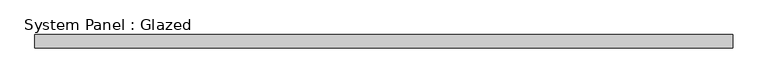
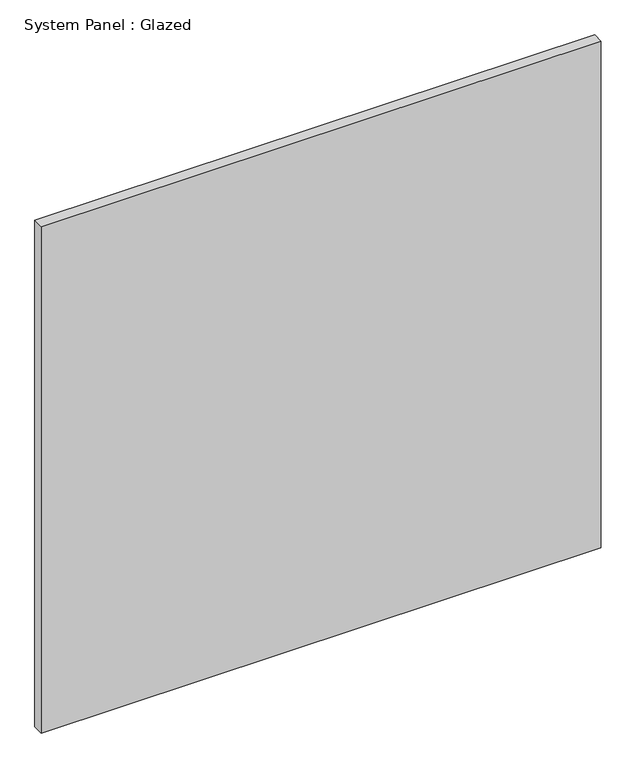
"""IFC4 building model written with IfcOpenShell, lengths in millimetres: plate geometry, System Panel : Glazed."""

from ifc_helpers import new_model, si_unit, origin, origin_with_axes, place, context, project, spatial, polyline, outline, extrude, source, transform, mapped, element, save


def system_panel_glazed_7e5d82eb(model_context):
    return source(origin(), model_context, "Body", "SweptSolid", [
        extrude(outline(polyline([(667.8083334, 19.05), (-667.8083334, 19.05), (-667.8083334, 44.45), (667.8083334, 44.45), (667.8083334, 19.05)])), origin_with_axes(), (0.0, 0.0, 1.0), 1276.35),
    ])


if __name__ == "__main__":
    model = new_model("IFC4")
    model_context = context("Model", 3, world=origin())
    ifc_project = project(units=[si_unit("LENGTHUNIT", "METRE", prefix="MILLI")], contexts=[model_context])
    site = spatial("IfcSite", under=ifc_project)
    building = spatial("IfcBuilding", under=site)
    placement = place(None, origin())
    system_panel_glazed_shape = system_panel_glazed_7e5d82eb(model_context)
    element("IfcPlate", 1, ObjectType="System Panel : Glazed", at=placement, inside=building, context=model_context, shape_type="MappedRepresentation", body=[
        mapped(system_panel_glazed_shape, transform((0.0, 0.0, 0.0), x_axis=(1.0, 0.0, 0.0), y_axis=(0.0, 1.0, 0.0), z_axis=(0.0, 0.0, 1.0))),
    ])
    save(model, "model.ifc")

# Revit data of these elements
# Type "System Panel : Glazed"
#   Construction Type Id = "GSP4R"
#   Analytic Construction = "1/8 in Pilkington single glazing"
#   Visual Light Transmittance = 0.9
#   Solar Heat Gain Coefficient = 0.86
#   Heat Transfer Coefficient (U) = 1.18115 BTU/(h·ft²·°F)
#   Define Thermal Properties by = 1
# Element 1 (IfcPlate, "System Panel : Glazed")
#   Materials on its faces: "Glass"
# Materials
#   "Glass": class "Glass", colour RGB 0 128 192, transparency 0.75, Description = "Soda Lime Glass", Cost = 0
